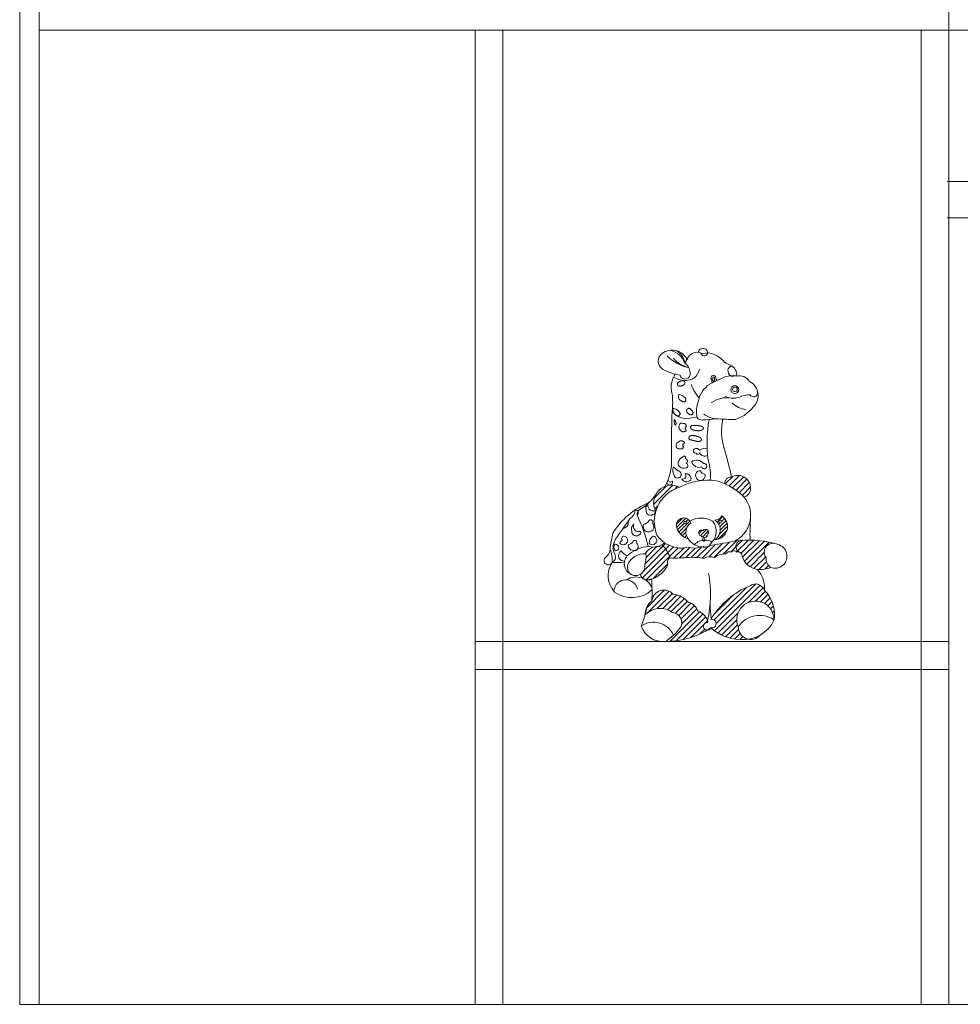
# Model space of a CAD drawing. Units: inches. Extents: x -17 to 1735, y -531 to 60.
# Tile 16 of 27: x 1734.74915 to 1734.789, y -150.26456 to -150.22283. Entities that reach past the tile are written whole.
import ezdxf

# ---------------------------------------------------------------- set-up
doc = ezdxf.new("R2010")
doc.units = ezdxf.units.IN
doc.header["$MEASUREMENT"] = 0
doc.layers.add('A-FURN', color=242, linetype='Continuous', lineweight=18, true_color=0xcd2027)
pattern_1 = [(45, (73.3040406, 53.313861), (-0.0030547, 0.0030547), [])]

# ---------------------------------------------------------------- blocks, each defined once
blk = doc.blocks.new('childrens_room_2')
h = blk.add_hatch()
h.set_pattern_fill('ANSI31', color=256, scale=0.03456, style=0)
h.set_pattern_definition(pattern_1)
h.paths.add_polyline_path([(72.7336, 53.4838, -0.002893), (72.7333, 53.4833, 0.264492), (72.7328, 53.4644, -0.250845), (72.7582, 53.4904, 0.383068)])
h.paths.add_polyline_path([(72.8213, 53.4858, -0.075102), (72.8281, 53.4795, 0.334621), (72.8348, 53.491, 0.539911), (72.8141, 53.5012, 0.440703), (72.807, 53.4941, -0.059176)])
h = blk.add_hatch()
h.set_pattern_fill('ANSI31', color=256, scale=0.0216, style=0)
h.set_pattern_definition([(45, (73.3040406, 53.3138612), (-0.001909188, 0.001909188), [])])
h.paths.add_polyline_path([(72.7704, 53.4516), (72.7694, 53.4539, 0.784014), (72.755, 53.4481, 0.284726), (72.7677, 53.4347, -0.439921)])
h.paths.add_polyline_path([(72.7631, 53.4522, -1), (72.766, 53.4522, -1)], flags=16)
h.paths.add_polyline_path([(72.7963, 53.434, 0.738442), (72.8039, 53.4595, -0.273758), (72.7959, 53.4549, -0.56758)])
h.paths.add_polyline_path([(72.8007, 53.4535, -1), (72.8036, 53.4535, -1)], flags=16)
h.paths.add_polyline_path([(72.7836, 53.4439, 1.14546), (72.7816, 53.438, 0.741718), (72.7888, 53.4397, 0.982448)])
h = blk.add_hatch()
h.set_pattern_fill('ANSI31', color=256, scale=0.03456, style=0)
h.set_pattern_definition(pattern_1)
h.paths.add_polyline_path([(72.7523, 53.4259, -0.083824), (72.7425, 53.4304, -0.045132), (72.7394, 53.4284, -0.146979), (72.748, 53.4138, -0.176175), (72.751, 53.4139, 0.01208), (72.7715, 53.4149, -0.040098), (72.7847, 53.4137, -0.236244), (72.7959, 53.4148, -0.155938), (72.8078, 53.4185, -0.361705), (72.8145, 53.4204, -0.568656), (72.8198, 53.4205, -0.133439), (72.8222, 53.4206, -0.661703), (72.8244, 53.4331, 0.012635), (72.8184, 53.4325, -0.020114), (72.7928, 53.428, -0.069751), (72.7885, 53.4262, -0.076899), (72.787, 53.4259, -0.093401), (72.7808, 53.426, -0.164353), (72.7679, 53.4258, -0.145726)])
h.paths.add_polyline_path([(72.748, 53.4138, 0.146979), (72.7394, 53.4284, -0.11109), (72.7307, 53.426, 0.202136), (72.7215, 53.4188, -0.008944), (72.7222, 53.4187, -0.08604), (72.7211, 53.4065, -0.30138), (72.7161, 53.3965, 0.180636), (72.7194, 53.3919, -0.023364), (72.7209, 53.3911, 0.234637), (72.7281, 53.3915, 0.229345), (72.7459, 53.4076, -0.451158)])
h.paths.add_polyline_path([(72.7516, 53.3751, 0.657875), (72.7285, 53.3679, 0.104837), (72.7232, 53.3611, -0.018431), (72.7211, 53.3527, -0.385559), (72.7509, 53.3554, -0.556882), (72.7594, 53.3395, -0.107757), (72.7429, 53.3243, 0.14192), (72.7883, 53.3366, -1.097392), (72.7889, 53.3446, 0.292101), (72.7781, 53.3569, 0.269374), (72.7679, 53.3663, 0.212687)])
h.paths.add_polyline_path([(72.7925, 53.349, 0.000847), (72.7926, 53.3481, -1.206105), (72.7919, 53.3389, 0.174787), (72.8234, 53.3263, 0.064596), (72.8328, 53.3267, -0.371526), (72.8215, 53.3401, -1.229609), (72.86, 53.3473, 0.245023), (72.85, 53.3792, 0.506577), (72.8345, 53.3844, 0.158953)])
h.paths.add_polyline_path([(72.8244, 53.4331, 0.661703), (72.8222, 53.4206, -0.336505), (72.8258, 53.4164, 0.302588), (72.8423, 53.4017, 0.119411), (72.8564, 53.404, -0.262234), (72.8515, 53.4147, -0.647325), (72.8601, 53.43, 0.075578)])
for p, q in [((72.0483, 55.5336), (72.0483, 52.9336)), ((72.0693, 55.2879), (72.0693, 52.9336)), ((73.0483, 52.9336), (73.0483, 54.0054)), ((72.0693, 53.9825), (73.1463, 53.9825)), ((72.5383, 52.9336), (72.5383, 53.9825)), ((72.5683, 53.9825), (72.5683, 52.9336)), ((73.0183, 53.9825), (73.0183, 52.9336)), ((73.0463, 53.8193), (74.0458, 53.8193)), ((73.0463, 53.7804), (74.0458, 53.7804)), ((72.5383, 53.3242), (72.5383, 53.2942)), ((73.0483, 53.3242), (72.5383, 53.3242)), ((73.0483, 53.3242), (73.0483, 53.2942)), ((73.0483, 53.2942), (72.5383, 53.2942)), ((72.0483, 52.9336), (74.0483, 52.9336))]:
    blk.add_line(p, q)
blk.add_lwpolyline([(72.7396, 53.6344, -0.434946), (72.7658, 53.6291, -0.335722), (72.7639, 53.6242, -0.233278), (72.7698, 53.6137, -0.98768), (72.7589, 53.6108, -0.084763), (72.7399, 53.6175, -0.503803)], format="xyb", close=True)
for points in [[(72.7536, 53.612, 0.204517), (72.7502, 53.5915)], [(72.7505, 53.5721, 0.013129), (72.7498, 53.5177, -0.121966), (72.7427, 53.4911, -0.121966)], [(72.7974, 53.564, 0.020824), (72.8187, 53.5633, 0.020824)], [(72.7255, 53.4737, 0.160243), (72.6866, 53.4409, 0.028551), (72.6838, 53.4263, -0.248833), (72.6799, 53.4156, 1.405296), (72.6859, 53.4093, 0.347898), (72.6885, 53.3775, 0.354759), (72.7287, 53.3797)], [(72.6989, 53.409, 0.035303), (72.6859, 53.4093, 0.035303)], [(72.713, 53.3806, 0.864233), (72.6878, 53.3791, 0.864233)]]:
    blk.add_lwpolyline(points, format="xyb")
for points in [[(72.7641, 53.6038), (72.7642, 53.6028), (72.7641, 53.6021), (72.7638, 53.6014), (72.7635, 53.6009), (72.7631, 53.6006), (72.7626, 53.6003), (72.7621, 53.6), (72.7616, 53.5998), (72.7611, 53.5996), (72.7606, 53.5995), (72.7601, 53.5993), (72.7597, 53.5992), (72.7593, 53.5992), (72.7589, 53.5991), (72.7585, 53.5991), (72.7581, 53.5992), (72.7578, 53.5993), (72.7575, 53.5994), (72.7572, 53.5996), (72.7569, 53.5998), (72.7567, 53.6001), (72.7565, 53.6003), (72.7563, 53.6006), (72.7562, 53.6009), (72.7562, 53.6012), (72.7562, 53.6015), (72.7563, 53.6019), (72.7564, 53.6022), (72.7565, 53.6025), (72.7567, 53.6028), (72.7569, 53.6031), (72.7572, 53.6033), (72.7575, 53.6036), (72.7579, 53.6038), (72.7583, 53.604), (72.7587, 53.6042), (72.7592, 53.6044), (72.7597, 53.6045), (72.7602, 53.6046), (72.7607, 53.6047), (72.7612, 53.6048), (72.7618, 53.6048), (72.7623, 53.6047), (72.7628, 53.6047), (72.7633, 53.6045), (72.7636, 53.6043), (72.7639, 53.6041), (72.7641, 53.6038)], [(72.7575, 53.5901), (72.7585, 53.59), (72.7595, 53.5898), (72.7603, 53.5895), (72.7609, 53.5892), (72.7615, 53.5889), (72.7621, 53.5885), (72.7625, 53.5882), (72.763, 53.5878), (72.7634, 53.5874), (72.7637, 53.5871), (72.7641, 53.5868), (72.7644, 53.5864), (72.7646, 53.5861), (72.7648, 53.5858), (72.765, 53.5854), (72.7652, 53.5851), (72.7652, 53.5847), (72.7653, 53.5844), (72.7652, 53.584), (72.7652, 53.5837), (72.7651, 53.5834), (72.7649, 53.5831), (72.7647, 53.5828), (72.7645, 53.5826), (72.7643, 53.5824), (72.764, 53.5823), (72.7637, 53.5822), (72.7634, 53.5821), (72.763, 53.5821), (72.7627, 53.5821), (72.7623, 53.5822), (72.7619, 53.5823), (72.7615, 53.5825), (72.7612, 53.5827), (72.7608, 53.5829), (72.7604, 53.5832), (72.76, 53.5835), (72.7596, 53.5838), (72.7592, 53.5842), (72.7588, 53.5845), (72.7583, 53.5849), (72.7579, 53.5853), (72.7576, 53.5858), (72.7573, 53.5864), (72.7571, 53.5871), (72.7571, 53.5879), (72.7572, 53.5889), (72.7575, 53.5901)], [(72.7511, 53.5751), (72.7522, 53.575), (72.7531, 53.5748), (72.7539, 53.5745), (72.7546, 53.5742), (72.7552, 53.5739), (72.7557, 53.5735), (72.7562, 53.5732), (72.7566, 53.5728), (72.757, 53.5725), (72.7574, 53.5721), (72.7577, 53.5718), (72.758, 53.5714), (72.7583, 53.5711), (72.7585, 53.5708), (72.7587, 53.5704), (72.7588, 53.5701), (72.7589, 53.5697), (72.7589, 53.5694), (72.7589, 53.569), (72.7588, 53.5687), (72.7587, 53.5684), (72.7586, 53.5681), (72.7584, 53.5678), (72.7582, 53.5676), (72.7579, 53.5674), (72.7576, 53.5673), (72.7573, 53.5672), (72.757, 53.5671), (72.7567, 53.5671), (72.7563, 53.5671), (72.7559, 53.5672), (72.7556, 53.5673), (72.7552, 53.5675), (72.7548, 53.5677), (72.7544, 53.5679), (72.7541, 53.5682), (72.7537, 53.5686), (72.7534, 53.5689), (72.753, 53.5693), (72.7527, 53.5697), (72.7524, 53.5702), (72.7521, 53.5707), (72.7519, 53.5712), (72.7516, 53.5718), (72.7514, 53.5725), (72.7513, 53.5733), (72.7512, 53.5742), (72.7511, 53.5751)], [(72.7672, 53.5747), (72.7676, 53.5751), (72.768, 53.5753), (72.7684, 53.5754), (72.7689, 53.5752), (72.7693, 53.575), (72.7698, 53.5747), (72.7702, 53.5744), (72.7706, 53.574), (72.771, 53.5737), (72.7714, 53.5733), (72.7717, 53.573), (72.772, 53.5727), (72.7723, 53.5723), (72.7725, 53.572), (72.7727, 53.5717), (72.7728, 53.5713), (72.7729, 53.571), (72.7729, 53.5706), (72.7729, 53.5703), (72.7728, 53.5699), (72.7727, 53.5696), (72.7726, 53.5693), (72.7724, 53.5691), (72.7722, 53.5688), (72.7719, 53.5686), (72.7716, 53.5685), (72.7713, 53.5684), (72.771, 53.5683), (72.7707, 53.5683), (72.7703, 53.5684), (72.77, 53.5684), (72.7696, 53.5685), (72.7692, 53.5687), (72.7688, 53.5689), (72.7685, 53.5692), (72.7681, 53.5695), (72.7677, 53.5698), (72.7674, 53.5701), (72.7671, 53.5705), (72.7667, 53.571), (72.7664, 53.5714), (72.7662, 53.5719), (72.766, 53.5724), (72.7659, 53.5729), (72.766, 53.5734), (72.7662, 53.5738), (72.7666, 53.5743), (72.7672, 53.5747)], [(72.7526, 53.5632), (72.7533, 53.5623), (72.7539, 53.5615), (72.7542, 53.5608), (72.7545, 53.5601), (72.7546, 53.5595), (72.7546, 53.5589), (72.7546, 53.5584), (72.7545, 53.558), (72.7545, 53.5577), (72.7544, 53.5575), (72.7544, 53.5573), (72.7543, 53.5573), (72.7543, 53.5573), (72.7542, 53.5573), (72.754, 53.5575), (72.7538, 53.5577), (72.7536, 53.5579), (72.7534, 53.5583), (72.7531, 53.5587), (72.7529, 53.5593), (72.7527, 53.56), (72.7526, 53.5609), (72.7525, 53.5619), (72.7526, 53.5632)], [(72.7596, 53.5593), (72.7588, 53.5584), (72.7582, 53.5576), (72.7578, 53.5568), (72.7576, 53.5561), (72.7575, 53.5554), (72.7576, 53.5547), (72.7578, 53.5541), (72.7581, 53.5536), (72.7584, 53.553), (72.7587, 53.5525), (72.7591, 53.552), (72.7595, 53.5515), (72.7599, 53.5511), (72.7604, 53.5508), (72.7608, 53.5505), (72.7612, 53.5503), (72.7616, 53.5501), (72.762, 53.5501), (72.7623, 53.55), (72.7627, 53.5501), (72.763, 53.5501), (72.7634, 53.5502), (72.7637, 53.5503), (72.764, 53.5503), (72.7643, 53.5504), (72.7646, 53.5505), (72.7649, 53.5506), (72.7652, 53.5507), (72.7654, 53.5508), (72.7655, 53.5509), (72.7656, 53.551), (72.7656, 53.5512), (72.7656, 53.5515), (72.7654, 53.5517), (72.7652, 53.552), (72.7651, 53.5523), (72.7649, 53.5526), (72.7647, 53.553), (72.7646, 53.5533), (72.7645, 53.5537), (72.7646, 53.554), (72.7647, 53.5543), (72.7648, 53.5546), (72.765, 53.555), (72.7652, 53.5553), (72.7654, 53.5556), (72.7655, 53.5559), (72.7656, 53.5563), (72.7656, 53.5566), (72.7656, 53.5569), (72.7655, 53.5573), (72.7653, 53.5576), (72.765, 53.5579), (72.7648, 53.5582), (72.7645, 53.5584), (72.7641, 53.5586), (72.7637, 53.5588), (72.7633, 53.5589), (72.7629, 53.559), (72.7623, 53.5591), (72.7618, 53.5591), (72.7611, 53.5592), (72.7604, 53.5592), (72.7596, 53.5593)], [(72.7716, 53.557), (72.7722, 53.5569), (72.7726, 53.5569), (72.773, 53.5568), (72.7734, 53.5568), (72.7737, 53.5568), (72.7739, 53.5568), (72.7741, 53.5567), (72.7744, 53.5567), (72.7746, 53.5567), (72.7747, 53.5567), (72.7749, 53.5567), (72.7751, 53.5567), (72.7752, 53.5567), (72.7754, 53.5567), (72.7755, 53.5567), (72.7757, 53.5567), (72.7758, 53.5567), (72.776, 53.5567), (72.7761, 53.5567), (72.7762, 53.5567), (72.7764, 53.5566), (72.7765, 53.5566), (72.7766, 53.5566), (72.7768, 53.5566), (72.7769, 53.5566), (72.777, 53.5566), (72.7771, 53.5566), (72.7773, 53.5566), (72.7774, 53.5566), (72.7775, 53.5566), (72.7776, 53.5566), (72.7778, 53.5566), (72.7779, 53.5566), (72.778, 53.5566), (72.7781, 53.5566), (72.7782, 53.5566), (72.7783, 53.5566), (72.7785, 53.5566), (72.7786, 53.5566), (72.7787, 53.5566), (72.7788, 53.5566), (72.7789, 53.5565), (72.779, 53.5565), (72.7791, 53.5565), (72.7792, 53.5565), (72.7793, 53.5565), (72.7794, 53.5565), (72.7795, 53.5565), (72.7797, 53.5565), (72.7798, 53.5564), (72.7799, 53.5564), (72.78, 53.5564), (72.7801, 53.5564), (72.7802, 53.5564), (72.7803, 53.5564), (72.7804, 53.5563), (72.7805, 53.5563), (72.7806, 53.5563), (72.7807, 53.5563), (72.7808, 53.5563), (72.7809, 53.5562), (72.7809, 53.5562), (72.781, 53.5562), (72.7811, 53.5562), (72.7812, 53.5561), (72.7813, 53.5561), (72.7814, 53.5561), (72.7815, 53.5561), (72.7816, 53.556), (72.7817, 53.556), (72.7817, 53.556), (72.7818, 53.5559), (72.7819, 53.5559), (72.782, 53.5559), (72.7821, 53.5559), (72.7821, 53.5558), (72.7822, 53.5558), (72.7823, 53.5558), (72.7824, 53.5557), (72.7824, 53.5557), (72.7825, 53.5557), (72.7826, 53.5556), (72.7826, 53.5556), (72.7827, 53.5556), (72.7828, 53.5555), (72.7828, 53.5555), (72.7829, 53.5554), (72.783, 53.5554), (72.783, 53.5554), (72.7831, 53.5553), (72.7831, 53.5553), (72.7832, 53.5552), (72.7832, 53.5552), (72.7833, 53.5552), (72.7833, 53.5551), (72.7834, 53.5551), (72.7834, 53.555), (72.7835, 53.555), (72.7835, 53.5549), (72.7836, 53.5549), (72.7836, 53.5549), (72.7836, 53.5548), (72.7837, 53.5548), (72.7837, 53.5547), (72.7837, 53.5547), (72.7838, 53.5546), (72.7838, 53.5546), (72.7838, 53.5545), (72.7839, 53.5545), (72.7839, 53.5544), (72.7839, 53.5544), (72.7839, 53.5543), (72.7839, 53.5543), (72.784, 53.5542), (72.784, 53.5542), (72.784, 53.5541), (72.784, 53.5541), (72.784, 53.554), (72.784, 53.554), (72.784, 53.5539), (72.784, 53.5539), (72.784, 53.5538), (72.784, 53.5538), (72.784, 53.5537), (72.784, 53.5537), (72.784, 53.5536), (72.784, 53.5536), (72.784, 53.5535), (72.784, 53.5535), (72.784, 53.5534), (72.784, 53.5534), (72.784, 53.5533), (72.784, 53.5533), (72.7839, 53.5532), (72.7839, 53.5532), (72.7839, 53.5531), (72.7839, 53.5531), (72.7839, 53.553), (72.7838, 53.553), (72.7838, 53.5529), (72.7838, 53.5529), (72.7837, 53.5528), (72.7837, 53.5528), (72.7837, 53.5527), (72.7836, 53.5527), (72.7836, 53.5526), (72.7836, 53.5526), (72.7835, 53.5525), (72.7835, 53.5525), (72.7834, 53.5524), (72.7834, 53.5524), (72.7833, 53.5523), (72.7833, 53.5523), (72.7832, 53.5523), (72.7832, 53.5522), (72.7831, 53.5522), (72.7831, 53.5521), (72.783, 53.5521), (72.7829, 53.5521), (72.7829, 53.552), (72.7828, 53.552), (72.7828, 53.5519), (72.7827, 53.5519), (72.7826, 53.5519), (72.7825, 53.5518), (72.7825, 53.5518), (72.7824, 53.5518), (72.7823, 53.5517), (72.7823, 53.5517), (72.7822, 53.5517), (72.7821, 53.5517), (72.782, 53.5516), (72.7819, 53.5516), (72.7818, 53.5516), (72.7818, 53.5515), (72.7817, 53.5515), (72.7816, 53.5515), (72.7815, 53.5515), (72.7814, 53.5515), (72.7813, 53.5514), (72.7812, 53.5514), (72.7811, 53.5514), (72.781, 53.5514), (72.7809, 53.5514), (72.7808, 53.5513), (72.7807, 53.5513), (72.7806, 53.5513), (72.7805, 53.5513), (72.7804, 53.5513), (72.7803, 53.5513), (72.7802, 53.5513), (72.7801, 53.5513), (72.78, 53.5512), (72.7799, 53.5512), (72.7798, 53.5512), (72.7797, 53.5512), (72.7795, 53.5512), (72.7794, 53.5512), (72.7793, 53.5512), (72.7792, 53.5512), (72.7791, 53.5512), (72.779, 53.5512), (72.7788, 53.5512), (72.7787, 53.5512), (72.7786, 53.5512), (72.7785, 53.5512), (72.7784, 53.5512), (72.7782, 53.5512), (72.7781, 53.5512), (72.778, 53.5512), (72.7779, 53.5512), (72.7777, 53.5512), (72.7776, 53.5512), (72.7775, 53.5512), (72.7774, 53.5512), (72.7772, 53.5512), (72.7771, 53.5513), (72.777, 53.5513), (72.7769, 53.5513), (72.7767, 53.5513), (72.7766, 53.5513), (72.7765, 53.5513), (72.7763, 53.5513), (72.7762, 53.5513), (72.7761, 53.5513), (72.7759, 53.5514), (72.7758, 53.5514), (72.7757, 53.5514), (72.7755, 53.5514), (72.7754, 53.5514), (72.7753, 53.5514), (72.7752, 53.5515), (72.775, 53.5515), (72.7749, 53.5515), (72.7748, 53.5515), (72.7746, 53.5515), (72.7745, 53.5516), (72.7744, 53.5516), (72.7742, 53.5516), (72.7741, 53.5516), (72.774, 53.5517), (72.7738, 53.5517), (72.7737, 53.5517), (72.7736, 53.5518), (72.7735, 53.5518), (72.7733, 53.5518), (72.7732, 53.5519), (72.7731, 53.5519), (72.773, 53.5519), (72.7728, 53.552), (72.7727, 53.552), (72.7726, 53.5521), (72.7725, 53.5521), (72.7724, 53.5522), (72.7723, 53.5522), (72.7722, 53.5523), (72.7721, 53.5523), (72.7719, 53.5524), (72.7718, 53.5525), (72.7717, 53.5525), (72.7716, 53.5526), (72.7715, 53.5527), (72.7715, 53.5527), (72.7714, 53.5528), (72.7713, 53.5529), (72.7712, 53.553), (72.7711, 53.553), (72.771, 53.5531), (72.771, 53.5532), (72.7709, 53.5533), (72.7708, 53.5534), (72.7707, 53.5535), (72.7707, 53.5536), (72.7706, 53.5537), (72.7706, 53.5538), (72.7705, 53.554), (72.7705, 53.5541), (72.7704, 53.5542), (72.7704, 53.5544), (72.7703, 53.5546), (72.7703, 53.5547), (72.7703, 53.5549), (72.7703, 53.5552), (72.7704, 53.5554), (72.7706, 53.5557), (72.7708, 53.5561), (72.7712, 53.5565), (72.7716, 53.557)], [(72.7691, 53.5416), (72.7696, 53.5415), (72.77, 53.5414), (72.7704, 53.5413), (72.7708, 53.5413), (72.7711, 53.5412), (72.7713, 53.5411), (72.7716, 53.5411), (72.7718, 53.541), (72.7719, 53.541), (72.7721, 53.541), (72.7723, 53.5409), (72.7725, 53.5409), (72.7726, 53.5408), (72.7728, 53.5408), (72.7729, 53.5408), (72.773, 53.5407), (72.7732, 53.5407), (72.7733, 53.5406), (72.7734, 53.5406), (72.7736, 53.5406), (72.7737, 53.5405), (72.7738, 53.5405), (72.774, 53.5405), (72.7741, 53.5404), (72.7742, 53.5404), (72.7743, 53.5404), (72.7744, 53.5403), (72.7746, 53.5403), (72.7747, 53.5403), (72.7748, 53.5402), (72.7749, 53.5402), (72.775, 53.5402), (72.7752, 53.5401), (72.7753, 53.5401), (72.7754, 53.5401), (72.7755, 53.54), (72.7756, 53.54), (72.7757, 53.54), (72.7758, 53.54), (72.7759, 53.5399), (72.776, 53.5399), (72.7762, 53.5399), (72.7763, 53.5399), (72.7764, 53.5398), (72.7765, 53.5398), (72.7766, 53.5398), (72.7767, 53.5398), (72.7768, 53.5398), (72.7769, 53.5397), (72.777, 53.5397), (72.7771, 53.5397), (72.7772, 53.5397), (72.7773, 53.5397), (72.7774, 53.5397), (72.7775, 53.5397), (72.7776, 53.5396), (72.7777, 53.5396), (72.7778, 53.5396), (72.7779, 53.5396), (72.778, 53.5396), (72.7781, 53.5396), (72.7782, 53.5396), (72.7783, 53.5396), (72.7784, 53.5396), (72.7785, 53.5396), (72.7786, 53.5396), (72.7787, 53.5396), (72.7788, 53.5396), (72.7789, 53.5396), (72.7789, 53.5396), (72.779, 53.5396), (72.7791, 53.5396), (72.7792, 53.5396), (72.7793, 53.5396), (72.7794, 53.5396), (72.7795, 53.5396), (72.7795, 53.5396), (72.7796, 53.5396), (72.7797, 53.5396), (72.7798, 53.5396), (72.7799, 53.5397), (72.7799, 53.5397), (72.78, 53.5397), (72.7801, 53.5397), (72.7802, 53.5397), (72.7802, 53.5397), (72.7803, 53.5397), (72.7804, 53.5398), (72.7804, 53.5398), (72.7805, 53.5398), (72.7806, 53.5398), (72.7806, 53.5398), (72.7807, 53.5399), (72.7808, 53.5399), (72.7808, 53.5399), (72.7809, 53.5399), (72.7809, 53.54), (72.781, 53.54), (72.781, 53.54), (72.7811, 53.5401), (72.7811, 53.5401), (72.7812, 53.5401), (72.7812, 53.5402), (72.7813, 53.5402), (72.7813, 53.5402), (72.7814, 53.5403), (72.7814, 53.5403), (72.7815, 53.5403), (72.7815, 53.5404), (72.7815, 53.5404), (72.7816, 53.5405), (72.7816, 53.5405), (72.7816, 53.5405), (72.7817, 53.5406), (72.7817, 53.5406), (72.7817, 53.5407), (72.7818, 53.5407), (72.7818, 53.5408), (72.7818, 53.5408), (72.7818, 53.5409), (72.7818, 53.5409), (72.7819, 53.5409), (72.7819, 53.541), (72.7819, 53.541), (72.7819, 53.5411), (72.7819, 53.5411), (72.7819, 53.5412), (72.7819, 53.5413), (72.7819, 53.5413), (72.782, 53.5414), (72.782, 53.5414), (72.782, 53.5415), (72.782, 53.5415), (72.782, 53.5416), (72.782, 53.5416), (72.7819, 53.5417), (72.7819, 53.5417), (72.7819, 53.5418), (72.7819, 53.5418), (72.7819, 53.5419), (72.7819, 53.542), (72.7819, 53.542), (72.7819, 53.5421), (72.7818, 53.5421), (72.7818, 53.5422), (72.7818, 53.5422), (72.7818, 53.5423), (72.7817, 53.5423), (72.7817, 53.5424), (72.7817, 53.5425), (72.7817, 53.5425), (72.7816, 53.5426), (72.7816, 53.5426), (72.7816, 53.5427), (72.7815, 53.5427), (72.7815, 53.5428), (72.7814, 53.5429), (72.7814, 53.5429), (72.7813, 53.543), (72.7813, 53.543), (72.7812, 53.5431), (72.7812, 53.5431), (72.7811, 53.5432), (72.7811, 53.5432), (72.781, 53.5433), (72.781, 53.5433), (72.7809, 53.5434), (72.7809, 53.5434), (72.7808, 53.5435), (72.7807, 53.5436), (72.7807, 53.5436), (72.7806, 53.5437), (72.7805, 53.5437), (72.7804, 53.5438), (72.7804, 53.5438), (72.7803, 53.5439), (72.7802, 53.5439), (72.7801, 53.5439), (72.7801, 53.544), (72.78, 53.544), (72.7799, 53.5441), (72.7798, 53.5441), (72.7797, 53.5442), (72.7796, 53.5442), (72.7795, 53.5443), (72.7794, 53.5443), (72.7794, 53.5444), (72.7793, 53.5444), (72.7792, 53.5445), (72.7791, 53.5445), (72.779, 53.5445), (72.7789, 53.5446), (72.7788, 53.5446), (72.7787, 53.5447), (72.7786, 53.5447), (72.7785, 53.5447), (72.7783, 53.5448), (72.7782, 53.5448), (72.7781, 53.5449), (72.778, 53.5449), (72.7779, 53.5449), (72.7778, 53.545), (72.7777, 53.545), (72.7776, 53.545), (72.7775, 53.5451), (72.7773, 53.5451), (72.7772, 53.5451), (72.7771, 53.5452), (72.777, 53.5452), (72.7769, 53.5452), (72.7768, 53.5453), (72.7766, 53.5453), (72.7765, 53.5453), (72.7764, 53.5454), (72.7763, 53.5454), (72.7761, 53.5454), (72.776, 53.5455), (72.7759, 53.5455), (72.7758, 53.5455), (72.7756, 53.5456), (72.7755, 53.5456), (72.7754, 53.5456), (72.7753, 53.5456), (72.7751, 53.5457), (72.775, 53.5457), (72.7749, 53.5457), (72.7747, 53.5457), (72.7746, 53.5458), (72.7745, 53.5458), (72.7743, 53.5458), (72.7742, 53.5458), (72.7741, 53.5458), (72.7739, 53.5459), (72.7738, 53.5459), (72.7737, 53.5459), (72.7736, 53.5459), (72.7734, 53.5459), (72.7733, 53.546), (72.7732, 53.546), (72.773, 53.546), (72.7729, 53.546), (72.7728, 53.546), (72.7726, 53.546), (72.7725, 53.546), (72.7724, 53.546), (72.7722, 53.546), (72.7721, 53.546), (72.772, 53.546), (72.7719, 53.546), (72.7717, 53.546), (72.7716, 53.546), (72.7715, 53.546), (72.7713, 53.546), (72.7712, 53.546), (72.7711, 53.546), (72.771, 53.546), (72.7709, 53.5459), (72.7707, 53.5459), (72.7706, 53.5459), (72.7705, 53.5458), (72.7704, 53.5458), (72.7703, 53.5458), (72.7702, 53.5457), (72.7701, 53.5457), (72.77, 53.5456), (72.7699, 53.5456), (72.7698, 53.5455), (72.7697, 53.5455), (72.7696, 53.5454), (72.7695, 53.5453), (72.7694, 53.5453), (72.7693, 53.5452), (72.7692, 53.5451), (72.7691, 53.545), (72.769, 53.5449), (72.7689, 53.5448), (72.7688, 53.5447), (72.7687, 53.5446), (72.7687, 53.5445), (72.7686, 53.5443), (72.7685, 53.5442), (72.7684, 53.544), (72.7684, 53.5437), (72.7684, 53.5435), (72.7684, 53.5431), (72.7686, 53.5427), (72.7688, 53.5422), (72.7691, 53.5416)], [(72.7558, 53.5321), (72.7553, 53.5332), (72.7549, 53.5342), (72.7548, 53.535), (72.7548, 53.5358), (72.7549, 53.5364), (72.7552, 53.537), (72.7555, 53.5376), (72.7559, 53.5381), (72.7564, 53.5385), (72.7569, 53.5389), (72.7574, 53.5393), (72.7579, 53.5396), (72.7584, 53.5399), (72.7589, 53.5401), (72.7594, 53.5402), (72.7598, 53.5403), (72.7603, 53.5404), (72.7606, 53.5403), (72.761, 53.5403), (72.7613, 53.5402), (72.7616, 53.54), (72.7619, 53.5399), (72.7622, 53.5397), (72.7625, 53.5395), (72.7628, 53.5394), (72.7631, 53.5392), (72.7633, 53.5391), (72.7636, 53.5389), (72.7637, 53.5388), (72.7638, 53.5386), (72.7639, 53.5384), (72.7638, 53.5383), (72.7637, 53.5381), (72.7635, 53.5378), (72.7633, 53.5376), (72.763, 53.5374), (72.7627, 53.5371), (72.7625, 53.5368), (72.7623, 53.5365), (72.7621, 53.5362), (72.7621, 53.5359), (72.7621, 53.5355), (72.7621, 53.5352), (72.7622, 53.5348), (72.7623, 53.5345), (72.7624, 53.5341), (72.7625, 53.5337), (72.7625, 53.5334), (72.7624, 53.5331), (72.7623, 53.5328), (72.762, 53.5325), (72.7618, 53.5322), (72.7615, 53.532), (72.7611, 53.5318), (72.7608, 53.5317), (72.7604, 53.5316), (72.76, 53.5315), (72.7595, 53.5315), (72.7591, 53.5315), (72.7586, 53.5316), (72.758, 53.5317), (72.7574, 53.5318), (72.7566, 53.532), (72.7558, 53.5321)], [(72.7694, 53.4539), (72.7704, 53.4516)]]:
    blk.add_lwpolyline(points)
for centre, radius in [((72.8178, 53.5954), 0.00428), ((72.818, 53.5956), 0.00251), ((72.7645, 53.4522), 0.00147), ((72.8022, 53.4535), 0.00147)]:
    blk.add_circle(centre, radius)
for centre, radius, start, end in [((72.7442, 53.6173), 0.0208, 19.3677, 76.9607), ((72.7472, 53.6221), 0.017, 10.4686, 61.4957), ((72.7836, 53.6346), 0.0052, 17.0582, 169.6177), ((72.7776, 53.6634), 0.0454, 223.9187, 257.4287), ((72.7724, 53.6452), 0.026, 217.5544, 260.3139), ((72.7508, 53.6353), 0.0174, 319.8372, 336.9559), ((72.7775, 53.624), 0.0117, 80.2872, 157.0274), ((72.7846, 53.6486), 0.0142, 248.7941, 286.7022), ((72.7789, 53.6321), 0.00341, 10.1715, 80.2872), ((72.7849, 53.6354), 0.00379, 226.0316, 11.2831), ((72.7845, 53.6063), 0.0291, 39.332, 81.7905), ((72.7651, 53.6203), 0.0151, 264.1992, 349.4859), ((72.8256, 53.6541), 0.0347, 237.6449, 248.8013), ((72.8165, 53.6156), 0.00605, 114.0711, 266.6654), ((72.809, 53.6115), 0.0109, 352.1221, 68.2777), ((72.7666, 53.6379), 0.0328, 243.1113, 265.1668), ((72.9364, 53.3151), 0.3211, 113.5954, 116.9651), ((72.7949, 53.6078), 0.00278, 19.8794, 183.48), ((72.7896, 53.605), 0.00358, 340.149, 45.5301), ((72.789, 53.6073), 0.00526, 336.7694, 13.2306), ((72.7952, 53.6075), 0.00136, 13.3956, 137.7028), ((72.7982, 53.6064), 0.00225, 140.4078, 247.8231), ((72.8001, 53.608), 0.00272, 165.1862, 252.6442), ((72.8166, 53.5637), 0.0465, 86.0919, 100.8297), ((72.8227, 53.5975), 0.0128, 33.2685, 102.9974), ((72.8182, 53.6189), 0.0506, 200.7513, 219.996), ((72.8056, 53.5782), 0.0274, 122.5549, 168.8868), ((72.794, 53.604), 0.00105, 189.4564, 33.6169), ((72.7937, 53.6038), 0.0014, 33.6169, 83.3096), ((72.8257, 53.5891), 0.0172, 324.4032, 63.5489), ((72.7498, 53.5914), 0.000389, 336.2142, 13.7858), ((72.6737, 53.5811), 0.0773, 353.3289, 7.3486), ((72.8097, 53.5574), 0.0293, 80.8993, 126.3262), ((72.8161, 53.6064), 0.0202, 244.3198, 296.9277), ((72.8353, 53.5543), 0.0356, 91.5102, 106.5289), ((72.8381, 53.5917), 0.00414, 206.0248, 10.7808), ((72.8071, 53.5721), 0.0306, 158.1672, 193.3831), ((72.8318, 53.5986), 0.0245, 225.7688, 266.334), ((72.805, 53.6036), 0.0425, 288.8754, 324.8659), ((72.7665, 53.5842), 0.0201, 217.1155, 271.0829), ((72.743, 53.7235), 0.1612, 278.5437, 282.2218), ((72.7825, 53.5697), 0.00703, 222.7092, 273.4754), ((72.7657, 53.8465), 0.2843, 273.4754, 276.4017), ((72.8, 53.5893), 0.0255, 232.4251, 264.0175), ((72.9358, 53.5382), 0.1478, 170.2416, 187.2737), ((72.8673, 53.5508), 0.0637, 168.386, 197.1225), ((72.7759, 53.5294), 0.00251, 123.6815, 277.4938), ((72.7765, 53.5279), 0.0041, 31.5764, 118.8826), ((72.7861, 53.5231), 0.00924, 76.9052, 131.1179), ((72.5471, 53.4522), 0.2713, 13.4551, 17.1225), ((72.7653, 53.5151), 0.00869, 112.5567, 168.4991), ((72.7634, 53.5224), 0.00154, 311.0838, 149.8819), ((72.7641, 53.5183), 0.00287, 301.6437, 85.2689), ((72.7781, 53.5279), 0.00208, 206.8158, 351.2233), ((72.7855, 53.5294), 0.0057, 199.4826, 303.1916), ((72.7632, 53.5084), 0.012, 161.527, 210.6873), ((72.8064, 53.571), 0.0802, 227.1355, 231.8563), ((72.7627, 53.5167), 0.00591, 178.0418, 286.5524), ((72.7649, 53.5135), 0.00253, 258.6878, 73.7986), ((72.7769, 53.5098), 0.00964, 38.1391, 125.2335), ((72.7796, 53.5204), 0.0087, 198.198, 287.5806), ((72.7849, 53.513), 0.00281, 198.125, 98.6881), ((72.7357, 53.5033), 0.0559, 354.4961, 16.8505), ((72.6506, 53.4733), 0.1659, 9.7038, 14.6881), ((72.7563, 53.5041), 0.00389, 207.0848, 82.5707), ((72.7613, 53.5028), 0.00394, 260.7401, 36.073), ((72.7658, 53.5017), 0.0056, 209.8272, 335.7659), ((72.7646, 53.4988), 0.00636, 5.4005, 90.928), ((72.7808, 53.5029), 0.0052, 90.2078, 14.3863), ((72.7867, 53.5105), 0.0063, 201.8232, 262.771), ((72.8138, 53.4944), 0.00681, 87.6563, 182.7892), ((72.8211, 53.4893), 0.0138, 6.9656, 120.4259), ((72.7496, 53.4734), 0.0191, 63.1365, 207.9925), ((72.7697, 53.4536), 0.0385, 107.4009, 203.7856), ((72.7478, 53.4957), 0.0031, 187.528, 22.6987), ((72.7486, 53.4984), 0.00252, 175, 323.7473), ((72.79, 53.4259), 0.0719, 83.7313, 116.2609), ((72.779, 53.4298), 0.0701, 52.9562, 74.4233), ((72.8238, 53.4897), 0.0111, 292.6671, 6.6724), ((72.6908, 53.5103), 0.0504, 298.7504, 328.1864), ((72.8039, 53.46), 0.031, 297.7676, 56.0037), ((72.7299, 53.4672), 0.00786, 133.0056, 198.8934), ((72.7304, 53.4709), 0.00614, 160.9395, 283.5279), ((73.2472, 53.06), 0.6717, 143.7731, 146.168), ((72.7101, 53.4515), 0.00714, 130.8814, 193.5906), ((72.6991, 53.4667), 0.0117, 302.7396, 356.2402), ((72.7108, 53.4628), 0.00318, 308.6378, 90.431), ((72.7201, 53.4608), 0.0074, 133.6767, 183.7648), ((72.5625, 53.3883), 0.1666, 13.2734, 25.6015), ((72.7271, 53.4648), 0.00466, 182.3027, 303.1348), ((72.7296, 53.4636), 0.00261, 271.6561, 32.7617), ((72.7629, 53.4493), 0.00797, 35.7576, 188.1454), ((72.7816, 53.4322), 0.0249, 60.6142, 119.4705), ((72.796, 53.4639), 0.00901, 269.3385, 330.5788), ((72.7962, 53.4479), 0.0139, 270.6829, 56.4578), ((73.0909, 53.4397), 0.2567, 175.8288, 181.4075), ((72.6921, 53.4587), 0.0142, 291.3099, 321.1843), ((72.7144, 53.4449), 0.00786, 133.0056, 198.8934), ((72.7148, 53.4487), 0.00614, 160.9395, 283.5279), ((72.7251, 53.4479), 0.00578, 151.4683, 44.8453), ((72.7191, 53.4578), 0.00723, 277.2847, 333.4973), ((72.7273, 53.4531), 0.00225, 328.8372, 139.298), ((72.7722, 53.4517), 0.0175, 191.5511, 255.1232), ((72.7768, 53.4419), 0.0116, 123.3845, 218.3674), ((72.7802, 53.4428), 0.0177, 309.6685, 39.3454), ((72.7899, 53.4443), 0.0122, 302.0395, 60.353), ((72.6978, 53.4331), 0.00467, 218.2088, 82.0096), ((72.6988, 53.435), 0.00277, 97.4409, 230.7618), ((72.7116, 53.4426), 0.00466, 182.3027, 303.1348), ((72.714, 53.4413), 0.00261, 271.6561, 32.7617), ((72.7345, 53.4301), 0.0089, 120.93, 179.2884), ((72.7292, 53.4331), 0.00467, 218.2088, 82.0096), ((72.7607, 53.4573), 0.0325, 216.2236, 254.9996), ((72.7822, 53.4411), 0.00313, 63.1898, 258.7044), ((72.7849, 53.4399), 0.00385, 209.6682, 355.9282), ((72.7862, 53.4417), 0.00334, 321.7607, 139.7316), ((72.7031, 53.4254), 0.0162, 148.2832, 211.8142), ((72.6925, 53.4255), 0.0048, 134.4509, 230.9601), ((72.6893, 53.4253), 0.00358, 273.1358, 92.2753), ((72.6975, 53.4294), 0.00346, 97.2315, 166.6474), ((72.7021, 53.4356), 0.00723, 277.2847, 333.4973), ((72.7096, 53.4286), 0.00662, 181.2281, 272.5271), ((72.7287, 53.3874), 0.0394, 95.8813, 127.7853), ((72.7103, 53.4309), 0.00225, 328.8372, 139.298), ((72.7097, 53.4263), 0.00428, 272.5271, 54.8996), ((72.7346, 53.4115), 0.015, 68.3817, 151.0388), ((72.7296, 53.4465), 0.0206, 256.0053, 308.6005), ((72.7194, 53.4067), 0.0295, 13.9016, 47.3472), ((72.7603, 53.452), 0.0273, 252.9499, 286.1144), ((72.7856, 53.4479), 0.0223, 216.1221, 265.0369), ((72.774, 53.445), 0.0202, 252.292, 289.6251), ((72.7851, 53.4194), 0.0139, 87.3294, 139.2105), ((72.7843, 53.4424), 0.0167, 257.9617, 300.6497), ((72.7842, 53.4336), 0.00149, 94.6886, 295.3234), ((72.7867, 53.431), 0.00513, 234.4745, 339.0794), ((72.7844, 53.4335), 0.00133, 290.0909, 71.3446), ((72.7867, 53.423), 0.0104, 50.4881, 95.5375), ((72.749, 53.7481), 0.3231, 277.7871, 282.3963), ((72.8321, 53.3141), 0.1193, 76.4063, 96.5901), ((72.8259, 53.4264), 0.00688, 85.6399, 253.4781), ((72.8592, 53.4204), 0.00962, 59.5281, 216.6639), ((72.861, 53.4161), 0.013, 249.3605, 75.9208), ((72.6476, 53.4114), 0.0383, 356.9508, 18.7175), ((72.6838, 53.4148), 0.00584, 290.5679, 20.3139), ((72.6996, 53.4164), 0.00678, 125.3969, 203.9684), ((72.7039, 53.4256), 0.00899, 203.7058, 261.8068), ((72.7114, 53.408), 0.0125, 123.1693, 239.0767), ((72.7207, 53.3993), 0.0195, 85.4457, 158.7197), ((72.6864, 53.4157), 0.0359, 345.1648, 4.8352), ((72.7411, 53.8382), 0.4244, 271.3399, 274.1084), ((72.7709, 53.3319), 0.083, 80.4075, 89.5925), ((72.7913, 53.4031), 0.0125, 68.7082, 121.8765), ((72.8077, 53.398), 0.0205, 89.6913, 125.1441), ((72.8123, 53.4154), 0.00546, 66.2431, 145.7844), ((72.8172, 53.4189), 0.00308, 31.1837, 149.6836), ((72.8212, 53.4162), 0.00454, 3.3835, 108.1793), ((72.8451, 53.4215), 0.02, 194.6231, 261.9639), ((72.8635, 53.4136), 0.012, 175, 233.7763), ((72.6992, 53.4178), 0.00711, 215.313, 269.7944), ((72.712, 53.4041), 0.00973, 166.6726, 224.1266), ((72.7111, 53.4053), 0.0101, 232.1978, 6.8326), ((72.7204, 53.4179), 0.0275, 286.2515, 337.9199), ((72.7497, 53.4098), 0.00437, 72.7283, 209.826), ((72.8446, 53.4318), 0.0302, 265.6451, 292.8831), ((72.7116, 53.3757), 0.018, 17.2035, 123.5302), ((72.724, 53.3986), 0.00817, 194.5417, 300.1174), ((72.6666, 53.375), 0.1251, 346.9377, 10.4621), ((72.8187, 53.3811), 0.0313, 356.5242, 40.9836), ((72.5628, 53.377), 0.166, 356.8626, 5.0196), ((72.8678, 53.3023), 0.0885, 112.0754, 148.9449), ((72.8403, 53.3761), 0.0101, 17.8921, 125.3549), ((72.7416, 53.3665), 0.0131, 40.5231, 173.8828), ((72.7499, 53.3523), 0.0228, 37.8128, 85.8414), ((72.8244, 53.3536), 0.0362, 350.0106, 45.0808), ((72.742, 53.352), 0.0209, 130.1826, 178.0612), ((72.7649, 53.3528), 0.0138, 17.0072, 77.3117), ((73.0435, 53.3787), 0.2527, 183.3018, 186.9468), ((72.84, 53.3477), 0.02, 358.8644, 202.3832), ((72.6082, 53.3851), 0.1175, 337.9143, 348.2033), ((72.7375, 53.3376), 0.0223, 52.9939, 137.3324), ((72.7502, 53.3448), 0.0106, 329.8311, 86.2816), ((72.7739, 53.3422), 0.0152, 8.9767, 74.1092), ((72.8443, 53.3249), 0.0274, 55.0525, 146.1951), ((72.7303, 53.3213), 0.0237, 24.1866, 124.0568), ((72.7403, 53.3486), 0.0244, 198.2423, 276.1681), ((72.7882, 53.3406), 0.00403, 80.0044, 334.9112), ((72.7931, 53.3435), 0.0047, 254.7496, 104.7895), ((72.8268, 53.3629), 0.0367, 264.6783, 334.9041), ((72.7163, 53.3697), 0.0526, 300.3904, 324.9915), ((72.7443, 53.4088), 0.0845, 269.0109, 304.2293), ((72.8251, 53.3763), 0.05, 228.3695, 268.027), ((72.835, 53.3399), 0.0134, 179.2335, 318.4944)]:
    blk.add_arc(centre, radius, start, end)

msp = doc.modelspace()

# ---------------------------------------------------------------- block references
at = {"layer": 'A-FURN', "xscale": 0.0393700787401575, "yscale": 0.0393700787401575, "zscale": 0.0393700787401575}
msp.add_blockref('childrens_room_2', (1731.912601, -152.348565), dxfattribs=at)

doc.saveas('drawing.dxf')
